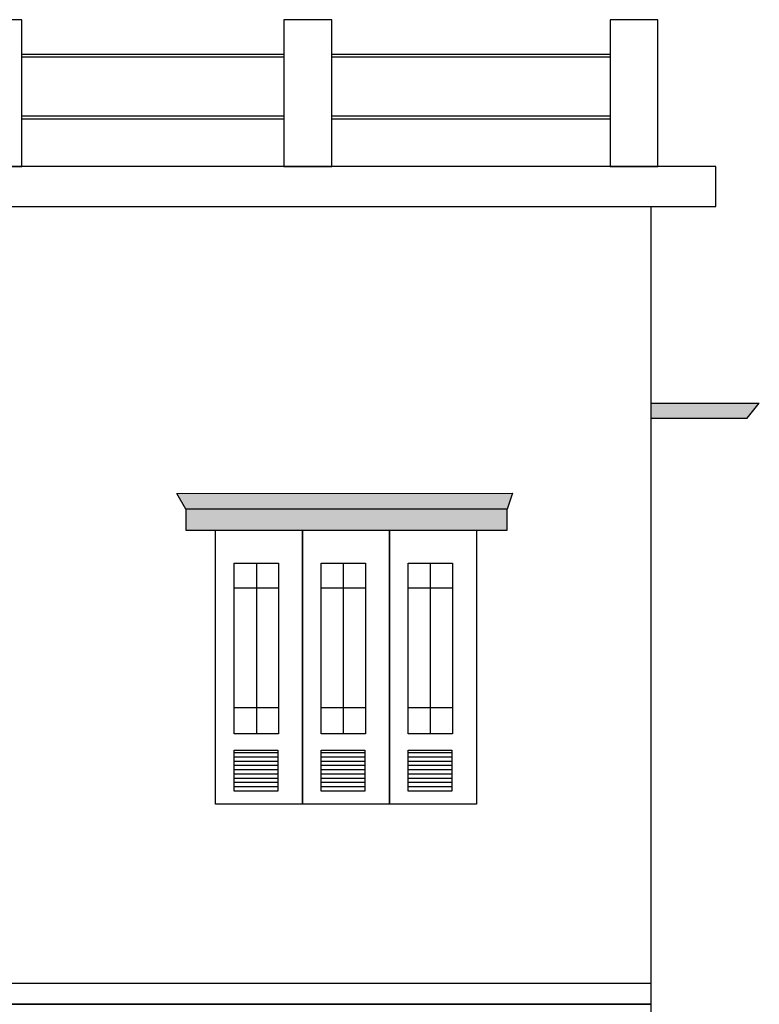
# Model space of a CAD drawing. Units: metres. Extents: x 10365 to 12529, y 3661 to 6248.
# Tile 9 of 9: x 11858 to 12379, y 5554 to 6248. Entities that reach past the tile are written whole.
import ezdxf

# ---------------------------------------------------------------- set-up
doc = ezdxf.new("R2010")
doc.units = ezdxf.units.M
doc.header["$MEASUREMENT"] = 0
doc.layers.add('A-ELEV', color=7, linetype='Continuous', lineweight=25)
doc.layers.add('A-ELEV-PATT', color=8, linetype='Continuous', lineweight=13)

msp = doc.modelspace()

# ---------------------------------------------------------------- hatches: boundary and pattern name
at = {"layer": 'A-ELEV-PATT'}
h = msp.add_hatch(color=256, dxfattribs=at)
h.dxf.hatch_style = 1
h.paths.add_polyline_path([(12379.49, 5977.79), (12303.22, 5977.79), (12303.22, 5967.13), (12370.96, 5967.13)])
h = msp.add_hatch(color=256, dxfattribs=at)
h.dxf.hatch_style = 1
h.paths.add_polyline_path([(12201.79, 5903.01), (11975.39, 5903.01), (11975.39, 5888.32), (12201.79, 5888.32)])
h.paths.add_polyline_path([(12205.55, 5914.48), (11968.98, 5914.12), (11975.39, 5903.01), (12201.79, 5903.01)])

# ---------------------------------------------------------------- linework, layer by layer
at = {"layer": 'A-ELEV'}
for p, q in [((11859.85, 6223.79), (12044.56, 6223.79)), ((11859.85, 6221.79), (12044.56, 6221.79)), ((12078.18, 6223.79), (12274.45, 6223.79)), ((12078.18, 6221.79), (12274.45, 6221.79)), ((11859.85, 6180.21), (12044.56, 6180.21)), ((11859.85, 6178.21), (12044.56, 6178.21)), ((12078.18, 6180.21), (12274.45, 6180.21)), ((12078.18, 6178.21), (12274.45, 6178.21)), ((11343.22, 6116.31), (12303.22, 6116.31)), ((12303.22, 5554.17), (12303.22, 6116.31)), ((12303.22, 5977.79), (12303.22, 5977.79)), ((12303.22, 5977.79), (12379.49, 5977.79)), ((12370.96, 5967.13), (12379.49, 5977.79)), ((12303.22, 5967.13), (12370.96, 5967.13)), ((11968.98, 5914.12), (12205.55, 5914.48)), ((11975.39, 5903.01), (11968.98, 5914.12)), ((12205.55, 5914.48), (12201.79, 5903.01)), ((12025.1, 5865.03), (12025.1, 5744.86)), ((12086.36, 5865.03), (12086.36, 5744.86)), ((12147.62, 5865.03), (12147.62, 5744.86)), ((12009.48, 5847.66), (12040.71, 5847.66)), ((12070.75, 5847.66), (12101.97, 5847.66)), ((12132.01, 5847.66), (12163.24, 5847.66)), ((12009.48, 5763.45), (12040.71, 5763.45)), ((12070.75, 5763.45), (12101.97, 5763.45)), ((12132.01, 5763.45), (12163.24, 5763.45)), ((12009.48, 5731.63), (12040.24, 5731.63)), ((12070.75, 5731.63), (12101.5, 5731.63)), ((12132.01, 5731.63), (12162.77, 5731.63)), ((12009.48, 5728.63), (12040.24, 5728.63)), ((12009.48, 5725.63), (12040.24, 5725.63)), ((12070.75, 5728.63), (12101.5, 5728.63)), ((12070.75, 5725.63), (12101.5, 5725.63)), ((12132.01, 5728.63), (12162.77, 5728.63)), ((12132.01, 5725.63), (12162.77, 5725.63)), ((12009.48, 5722.63), (12040.24, 5722.63)), ((12009.48, 5719.63), (12040.24, 5719.63)), ((12070.75, 5722.63), (12101.5, 5722.63)), ((12070.75, 5719.63), (12101.5, 5719.63)), ((12132.01, 5722.63), (12162.77, 5722.63)), ((12132.01, 5719.63), (12162.77, 5719.63)), ((12009.48, 5716.63), (12040.24, 5716.63)), ((12009.48, 5713.63), (12040.24, 5713.63)), ((12009.48, 5713.63), (12040.24, 5713.63)), ((12070.75, 5716.63), (12101.5, 5716.63)), ((12070.75, 5713.63), (12101.5, 5713.63)), ((12070.75, 5713.63), (12101.5, 5713.63)), ((12132.01, 5716.63), (12162.77, 5716.63)), ((12132.01, 5713.63), (12162.77, 5713.63)), ((12132.01, 5713.63), (12162.77, 5713.63)), ((12009.48, 5710.63), (12040.24, 5710.63)), ((12009.48, 5707.63), (12040.24, 5707.63)), ((12070.75, 5710.63), (12101.5, 5710.63)), ((12070.75, 5707.63), (12101.5, 5707.63)), ((12132.01, 5710.63), (12162.77, 5710.63)), ((12132.01, 5707.63), (12162.77, 5707.63)), ((11343.22, 5569.17), (12303.22, 5569.17)), ((12303.22, 5554.17), (11343.22, 5554.17)), ((11343.22, 5554.17), (12303.22, 5554.17)), ((12303.22, 4875.44), (12303.22, 5554.17))]:
    msp.add_line(p, q, dxfattribs=at)
for points in [[(11826.23, 6144.7), (11826.23, 6144.7), (11859.85, 6144.7), (11859.85, 6144.7), (11859.85, 6248.06), (11859.85, 6248.06), (11826.23, 6248.06), (11826.23, 6248.06)], [(12044.56, 6144.7), (12044.56, 6144.7), (12078.18, 6144.7), (12078.18, 6144.7), (12078.18, 6248.06), (12078.18, 6248.06), (12044.56, 6248.06), (12044.56, 6248.06)], [(12274.45, 6144.7), (12274.45, 6144.7), (12308.07, 6144.7), (12308.07, 6144.7), (12308.07, 6248.06), (12308.07, 6248.06), (12274.45, 6248.06), (12274.45, 6248.06)], [(11302.77, 6116.31), (11302.77, 6116.31), (12348.78, 6116.31), (12348.78, 6116.31), (12348.78, 6144.7), (12348.78, 6144.7), (11302.77, 6144.7), (11302.77, 6144.7)], [(11975.39, 5888.32), (11975.39, 5888.32), (12201.79, 5888.32), (12201.79, 5888.32), (12201.79, 5903.01), (12201.79, 5903.01), (11975.39, 5903.01), (11975.39, 5903.01)], [(11996.37, 5888.32), (11996.37, 5888.32), (12057.63, 5888.32), (12057.63, 5888.32), (12057.63, 5695.23), (12057.63, 5695.23), (11996.37, 5695.23), (11996.37, 5695.23)], [(12057.63, 5888.32), (12057.63, 5888.32), (12118.89, 5888.32), (12118.89, 5888.32), (12118.89, 5695.23), (12118.89, 5695.23), (12057.63, 5695.23), (12057.63, 5695.23)], [(12118.89, 5888.32), (12118.89, 5888.32), (12180.16, 5888.32), (12180.16, 5888.32), (12180.16, 5695.23), (12180.16, 5695.23), (12118.89, 5695.23), (12118.89, 5695.23)], [(12009.48, 5865.03), (12009.48, 5865.03), (12040.71, 5865.03), (12040.71, 5865.03), (12040.71, 5744.86), (12040.71, 5744.86), (12009.48, 5744.86), (12009.48, 5744.86)], [(12070.75, 5865.03), (12070.75, 5865.03), (12101.97, 5865.03), (12101.97, 5865.03), (12101.97, 5744.86), (12101.97, 5744.86), (12070.75, 5744.86), (12070.75, 5744.86)], [(12132.01, 5865.03), (12132.01, 5865.03), (12163.24, 5865.03), (12163.24, 5865.03), (12163.24, 5744.86), (12163.24, 5744.86), (12132.01, 5744.86), (12132.01, 5744.86)], [(12009.48, 5733.31), (12009.48, 5733.31), (12040.24, 5733.31), (12040.24, 5733.31), (12040.24, 5704.34), (12040.24, 5704.34), (12009.48, 5704.34), (12009.48, 5704.34)], [(12070.75, 5733.31), (12070.75, 5733.31), (12101.5, 5733.31), (12101.5, 5733.31), (12101.5, 5704.34), (12101.5, 5704.34), (12070.75, 5704.34), (12070.75, 5704.34)], [(12132.01, 5733.31), (12132.01, 5733.31), (12162.77, 5733.31), (12162.77, 5733.31), (12162.77, 5704.34), (12162.77, 5704.34), (12132.01, 5704.34), (12132.01, 5704.34)]]:
    msp.add_lwpolyline(points, close=True, dxfattribs=at)

doc.saveas('drawing.dxf')
